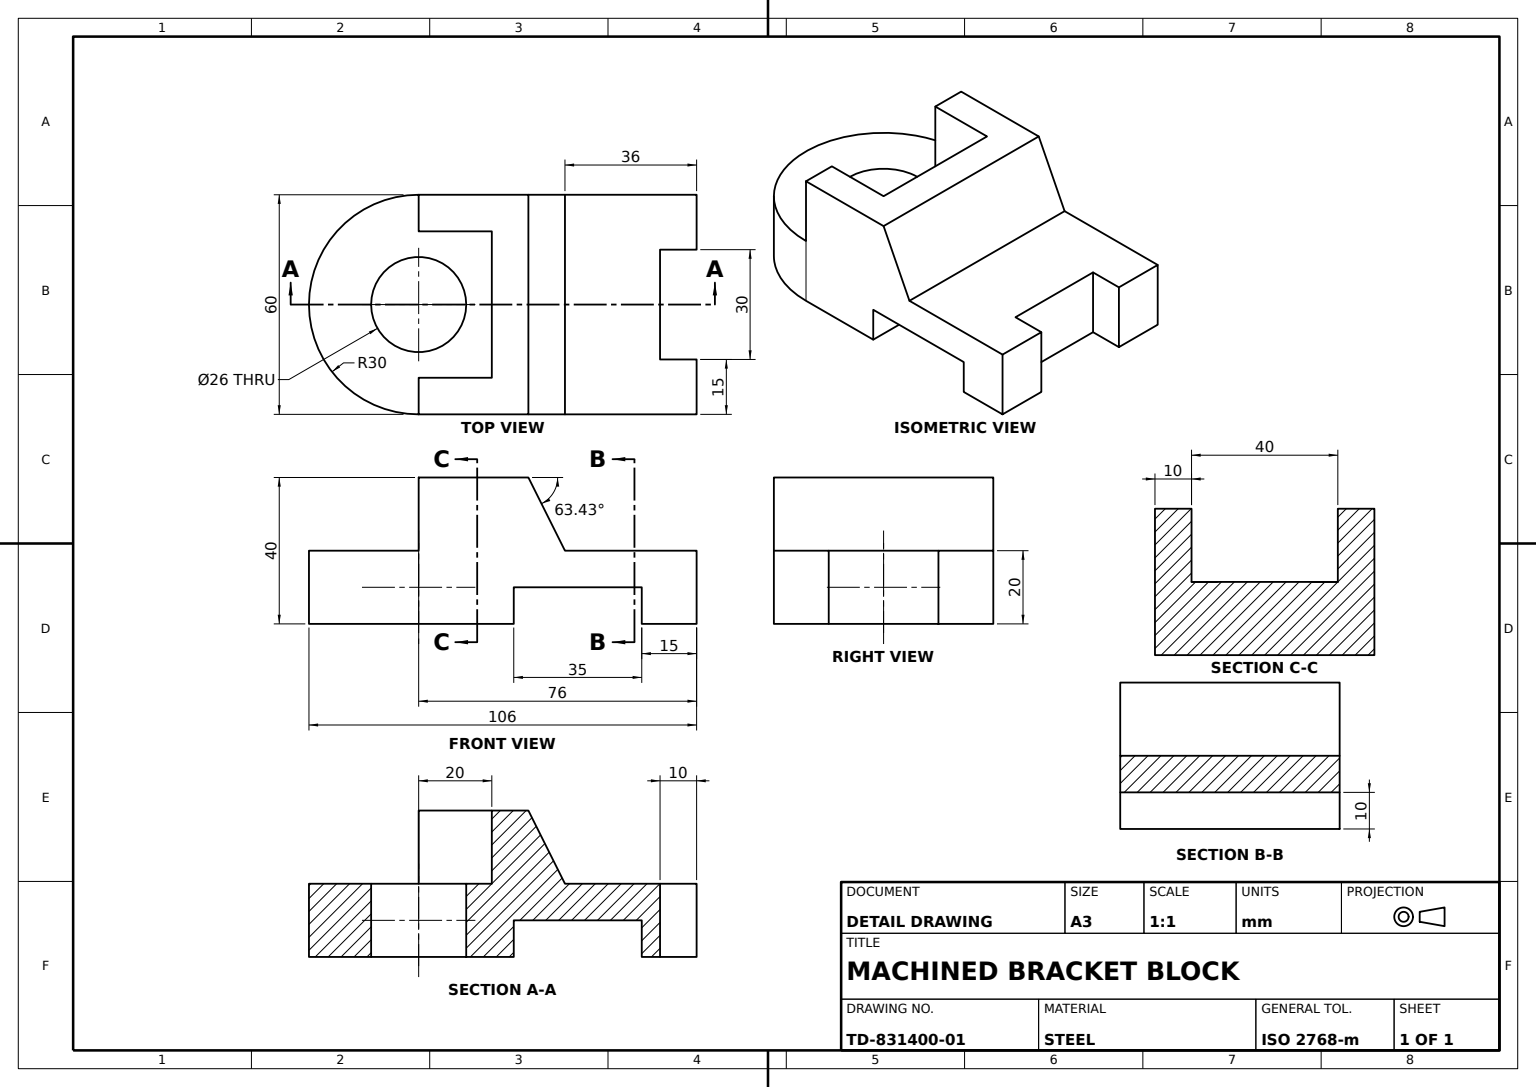
from build123d import *

# Parameters (mm, degrees)
BASE_PLATE_PROFILE_SKETCH_R   = 30
BASE_PLATE_PROFILE_SKETCH_R_2 = 13
BASE_PLATE_DEPTH              = 20
BASE_SLOT_CUT_REACH           = 100.874
BASE_SLOT_SKETCH_W            = 35
BASE_SLOT_SKETCH_H            = 10
BORE_CUT_REACH                = 86.119
BORE_SKETCH_W                 = 30
BORE_SKETCH_H                 = 10
UPRIGHT_BLOCK_DEPTH           = 30
UPRIGHT_BLOCK_DEPTH_BACK      = 30
UPRIGHT_POCKET_SKETCH_W       = 40
UPRIGHT_POCKET_SKETCH_H       = 20
UPRIGHT_POCKET_CUT_DEPTH      = 20


with BuildPart() as part:
    # Base Plate Profile Sketch → Base Plate (new body)
    # profile 1 of 2: a face of its own
    with BuildSketch(Plane(origin=(0, 0, 0), x_dir=(0, 0, -1), z_dir=(0, -1, 0))):
        with BuildLine():
            Line((76, 30), (0, 30))
            ThreePointArc((0, 30), (21.213203436, 21.213203436), (30, 0))
            ThreePointArc((30, 0), (21.213203436, -21.213203436), (0, -30))
            Line((0, -30), (76, -30))
            Line((76, -30), (76, 30))
        make_face()
    # profile 2 of 2: a face of its own
    with BuildSketch(Plane(origin=(0, 0, 0), x_dir=(0, 0, -1), z_dir=(0, -1, 0))):
        Circle(BASE_PLATE_PROFILE_SKETCH_R)
        with Locations(Location((0, 0, 0), (0, 0, 180))):
            Circle(BASE_PLATE_PROFILE_SKETCH_R_2, mode=Mode.SUBTRACT)
    extrude(amount=-BASE_PLATE_DEPTH)

    # Base Slot Sketch → Base Slot Cut (cut, up to next)
    with BuildSketch(Plane(origin=(30, 0, 0), x_dir=(0, 0, -1), z_dir=(1, 0, 0)), mode=Mode.PRIVATE) as base_slot_cut_sk1:
        with Locations((43.5, 5)):
            Rectangle(BASE_SLOT_SKETCH_W, BASE_SLOT_SKETCH_H)
    base_slot_cut_tool1 = extrude(base_slot_cut_sk1.sketch, amount=-BASE_SLOT_CUT_REACH, mode=Mode.PRIVATE) & part.part
    add(base_slot_cut_tool1.solids().sort_by_distance((30, 5, -43.5))[0], mode=Mode.SUBTRACT)

    # Bore Sketch → Bore Cut (cut, up to next)
    with BuildSketch(Plane(origin=(0, 20, 0), x_dir=(1, 0, 0), z_dir=(0, 1, 0)), mode=Mode.PRIVATE) as bore_cut_sk1:
        with Locations((0, 71)):
            Rectangle(BORE_SKETCH_W, BORE_SKETCH_H)
    bore_cut_tool1 = extrude(bore_cut_sk1.sketch, amount=-BORE_CUT_REACH, mode=Mode.PRIVATE) & part.part
    add(bore_cut_tool1.solids().sort_by_distance((0, 20, -71))[0], mode=Mode.SUBTRACT)

    # Upright Block Profile Sketch → Upright Block (add, two sides: drawn at the far end of the back side and taken through both)
    with BuildSketch(Plane(origin=(0, 0, 0), x_dir=(0, 0, -1), z_dir=(1, 0, 0)).offset(-UPRIGHT_BLOCK_DEPTH_BACK)):
        Polygon((0, 20), (0, 40), (30, 40), (40, 20), align=None)
    extrude(amount=UPRIGHT_BLOCK_DEPTH + UPRIGHT_BLOCK_DEPTH_BACK)

    # Upright Pocket Sketch → Upright Pocket Cut (cut)
    with BuildSketch(Plane(origin=(0, 40, 0), x_dir=(1, 0, 0), z_dir=(0, 1, 0))):
        with Locations((0, 10)):
            Rectangle(UPRIGHT_POCKET_SKETCH_W, UPRIGHT_POCKET_SKETCH_H)
    extrude(amount=-UPRIGHT_POCKET_CUT_DEPTH, mode=Mode.SUBTRACT)


solid = part.part
